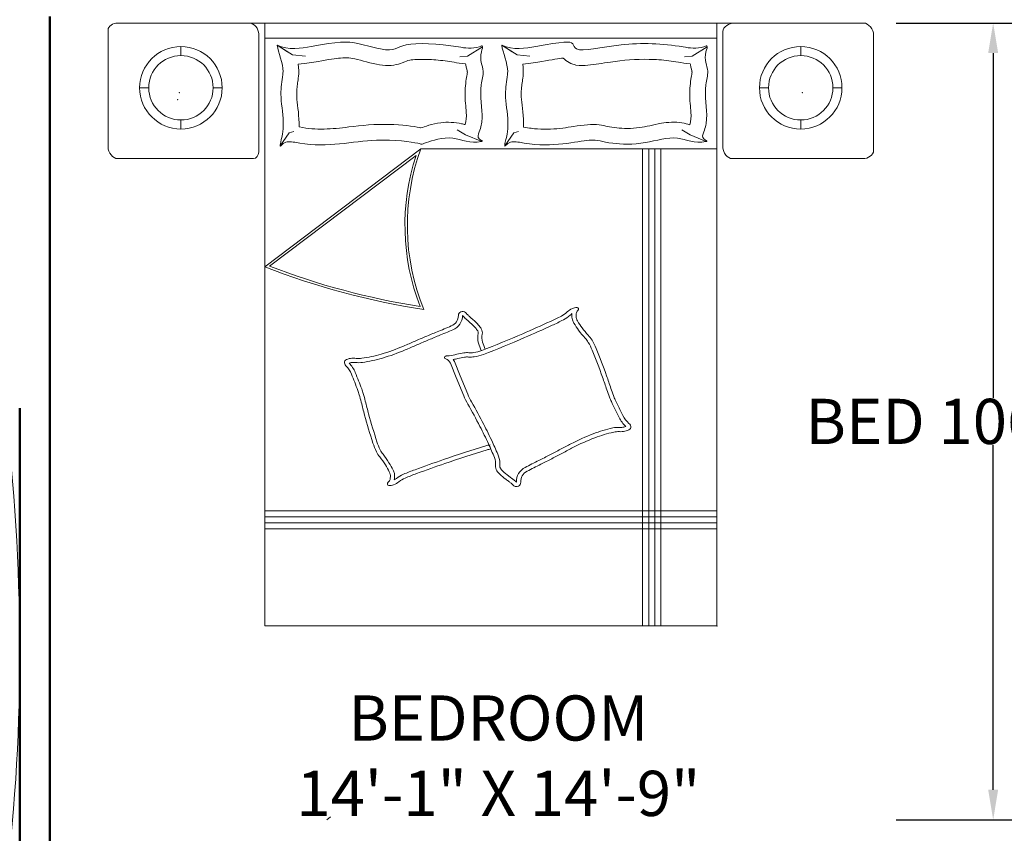
# Model space of a CAD drawing. Units: inches. Extents: x -466983 to 1020, y 324 to 318697.
# Tile 95 of 97: x 810 to 940, y 898 to 1006. Entities that reach past the tile are written whole.
import ezdxf

# ---------------------------------------------------------------- set-up
doc = ezdxf.new("R2010")
doc.units = ezdxf.units.IN
doc.header["$MEASUREMENT"] = 0
for name, color, linetype, lineweight in [('A-ANNO-DIMS', 2, 'Continuous', 18), ('A-AREA-IDEN', 7, 'Continuous', 25), ('A-FLOR-PATT', 252, 'Continuous', 13), ('A-FURN', 8, 'Continuous', 18), ('A-WALL', 7, 'Continuous', 50)]:
    doc.layers.add(name, color=color, linetype=linetype, lineweight=lineweight)
doc.styles.get("Standard").update_dxf_attribs({"font": 'arial.ttf'})
doc.dimstyles.get("Standard").update_dxf_attribs({"dimtxt": 6, "dimasz": 4, "dimexe": 3, "dimexo": 3, "dimgap": 0.09, "dimtad": 0, "dimtih": 1, "dimtoh": 1, "dimdec": 1, "dimzin": 0, "dimdsep": 46, "dimlunit": 3, "dimtxsty": 'Standard', "dimcen": 0.09, "dimadec": 0, "dimazin": 0, "dimtfac": 1, "dimtdec": 1, "dimtofl": 0, "dimtmove": 0, "dimatfit": 3, "dimfxl": 1, "dimtolj": 1, "dimtzin": 0, "dimarcsym": 0})

# ---------------------------------------------------------------- blocks, each defined once
blk = doc.blocks.new('A$C05F852CF')
for p, q in [((0.0306, 3.0783), (0.4692, 3.0783)), ((0.4692, 3.0783), (2.0768, 3.0783)), ((0.52, 3.0783), (0.52, 1.0783)), ((2.02, 3.0783), (2.02, 1.0783)), ((2.0768, 3.0783), (2.5066, 3.0783)), ((0, 3.0548), (0, 2.6659)), ((0.5, 3.0423), (0.5, 2.6496)), ((2.04, 3.05), (2.04, 2.6642)), ((2.54, 2.6547), (2.54, 3.0393)), ((0.52, 3.0283), (2.02, 3.0283)), ((0.2418, 2.9702), (0.2418, 3.0002)), ((0.5609, 3.0045), (0.5953, 2.9829)), ((0.5609, 3.0045), (0.6121, 2.9725)), ((1.2427, 2.9995), (1.1927, 2.9682)), ((2.2982, 2.9702), (2.2982, 3.0002)), ((0.6121, 2.9725), (0.6546, 2.9682)), ((1.1927, 2.9682), (1.1672, 2.9661)), ((0.1349, 2.8634), (0.1049, 2.8634)), ((0.3487, 2.8634), (0.3787, 2.8634)), ((2.1913, 2.8634), (2.1613, 2.8634)), ((2.4051, 2.8634), (2.4351, 2.8634)), ((0.2418, 2.7265), (0.2418, 2.7565)), ((2.2982, 2.7265), (2.2982, 2.7565)), ((0.5711, 2.6712), (0.6015, 2.7135)), ((0.6015, 2.7135), (0.6164, 2.7178)), ((1.1864, 2.7072), (1.1588, 2.7242)), ((1.2397, 2.6852), (1.1864, 2.7072)), ((1.0379, 2.6608), (0.52, 2.2697)), ((2.02, 2.6608), (1.0379, 2.6608)), ((1.7737, 2.6608), (1.7737, 1.0783)), ((1.7937, 2.6608), (1.7937, 1.0783)), ((1.8137, 2.6608), (1.8137, 1.0783)), ((1.8337, 2.6608), (1.8337, 1.0783)), ((0.0322, 2.6283), (0.4826, 2.6283)), ((2.0707, 2.6283), (2.5056, 2.6283)), ((0.52, 1.4597), (2.02, 1.4597)), ((0.52, 1.4397), (2.02, 1.4397)), ((0.52, 1.4197), (2.02, 1.4197)), ((0.52, 1.3997), (2.02, 1.3997)), ((0.52, 1.0783), (2.02, 1.0783)), ((0.726, 0.4346), (0.7377, 0.4444))]:
    blk.add_line(p, q)
for points in [[(1.3405, 2.9829), (1.306, 3.0045), (1.3573, 2.9725), (1.3998, 2.9682)], [(1.9879, 2.9995), (1.9379, 2.9682), (1.9124, 2.9661)], [(1.3162, 2.6712), (1.3467, 2.7135), (1.3616, 2.7178)], [(1.9848, 2.6852), (1.9315, 2.7072), (1.9039, 2.7242)]]:
    blk.add_lwpolyline(points)
for points in [[(1.0353, 2.1379, -0.173032), (1.022, 2.6388), (0.536, 2.2719, 0.053888)], [(1.7081, 1.7759, 0.101392), (1.7282, 1.7501, -0.223768), (1.7345, 1.736, -0.25558), (1.7315, 1.7308, -0.081563), (1.7151, 1.724, -0.071805), (1.6967, 1.7225, 0.069985), (1.6778, 1.7209, 0.03546), (1.6148, 1.7021, 0.029432), (1.5425, 1.6697, 0.001554), (1.5078, 1.6515, -0.00152), (1.4724, 1.6329, -0.004735), (1.4356, 1.6142, 0.00382), (1.3901, 1.5911, 0.296001), (1.3692, 1.5546, -0.649774), (1.3468, 1.5431, -0.02319), (1.3416, 1.5477, 0.0288), (1.3374, 1.5514, 0.005727), (1.3298, 1.557, -0.004358), (1.3198, 1.5645, -0.027528), (1.3001, 1.5812, -0.046214), (1.29, 1.5928, -0.194121), (1.2856, 1.6105, 0.133719), (1.2823, 1.6363, 0.011505), (1.2622, 1.682, 0.008882), (1.2338, 1.7401, 0.012426), (1.1937, 1.8139, -0.033612), (1.1801, 1.8418), (1.1552, 1.9026), (1.1361, 1.9495, 0.224341), (1.1204, 1.9638, -0.722772), (1.1202, 1.9734, -0.103513), (1.1242, 1.9739, 0.053465), (1.132, 1.9742, 0.030109), (1.1569, 1.9792, -0.031436), (1.1808, 1.984, -0.05324), (1.1971, 1.9844, 0.05518), (1.2128, 1.9849, 0.056271), (1.2402, 1.992, 0.0108), (1.3759, 2.0475, 0.00456), (1.4675, 2.0883, 0.01125), (1.5041, 2.106, 0.069394), (1.5235, 2.1196, -0.079756), (1.5405, 2.1311, -0.106399), (1.5562, 2.1345, -0.328642), (1.5608, 2.1312, -0.299547), (1.5587, 2.124, 0.189917), (1.5536, 2.1141, 0.033518), (1.5531, 2.1029, 0.075627), (1.554, 2.0981, 0.053489), (1.5579, 2.0898, 0.017838), (1.5727, 2.0672, 0.038394), (1.5932, 2.0425, -0.059529), (1.6058, 2.026, -0.035943), (1.6193, 1.9987, -0.011245), (1.6541, 1.9079, -0.006203), (1.6684, 1.8661, 0.010783), (1.6769, 1.8422, 0.019485), (1.6828, 1.8283, 0.005062)], [(1.6953, 1.7695, 0.098587), (1.7181, 1.7399, -0.040378), (1.7118, 1.7379, -0.071805), (1.6975, 1.7367, 0.069985), (1.6747, 1.7349, 0.03546), (1.6097, 1.7154, 0.029432), (1.5359, 1.6824, 0.001554), (1.5012, 1.6641, -0.00152), (1.4658, 1.6456, -0.004735), (1.4293, 1.627, 0.00382), (1.3835, 1.6038, 0.289814), (1.3549, 1.555, -0.018279), (1.3515, 1.5579, 0.0288), (1.3461, 1.5627, 0.005727), (1.3382, 1.5686, -0.004358), (1.3285, 1.5758, -0.027528), (1.31, 1.5916, -0.046214), (1.3016, 1.6012, -0.194121), (1.2997, 1.6085, 0.133719), (1.2955, 1.6417, 0.011505), (1.2752, 1.6881, 0.008882), (1.2465, 1.7466, 0.012426), (1.2061, 1.821, -0.033612), (1.1933, 1.8472), (1.1684, 1.908), (1.1493, 1.9549, 0.051417), (1.1455, 1.962, 0.017208), (1.1606, 1.9654, -0.031436), (1.1827, 1.9698, -0.05324), (1.196, 1.9702, 0.05518), (1.2149, 1.9708, 0.056271), (1.2453, 1.9787, 0.0108), (1.3816, 2.0344, 0.00456), (1.4734, 2.0753, 0.01125), (1.5106, 2.0933, 0.069394), (1.5332, 2.1091, -0.038161), (1.5392, 2.114, 0.029361), (1.5389, 2.1025, 0.075627), (1.5405, 2.0934, 0.053489), (1.5457, 2.0824, 0.017838), (1.5611, 2.0589, 0.038394), (1.583, 2.0326, -0.059529), (1.5935, 2.0187, -0.035943), (1.6061, 1.9933, -0.011245), (1.6406, 1.9031, -0.006203), (1.6549, 1.8617, 0.010783), (1.6635, 1.8371, 0.019485), (1.6699, 1.8222, 0.005062)]]:
    blk.add_lwpolyline(points, format="xyb", close=True)
for points in [[(1.27, 1.665, 0.025626), (1.2575, 1.662, 0.0108), (1.1179, 1.617, 0.00456), (1.0234, 1.5834, 0.01125), (0.9856, 1.5685, 0.069394), (0.9653, 1.5565, -0.079756), (0.9474, 1.5464, -0.106399), (0.9315, 1.5441, -0.328642), (0.9272, 1.5478, -0.299547), (0.9298, 1.5548, 0.189917), (0.9357, 1.5643, 0.033518), (0.9369, 1.5754, 0.075627), (0.9364, 1.5803, 0.053489), (0.9332, 1.5888, 0.017838), (0.9202, 1.6125, 0.038394), (0.9016, 1.6387, -0.059529), (0.8903, 1.6561, -0.035943), (0.8789, 1.6844, -0.011245), (0.8512, 1.7776, -0.006203), (0.8402, 1.8203, 0.010783), (0.8336, 1.8448, 0.019485), (0.8287, 1.8592, 0.005062), (0.8076, 1.9133, 0.101392), (0.7895, 1.9406, -0.223768), (0.7843, 1.9551, -0.25558), (0.7876, 1.9601, -0.081563), (0.8046, 1.9656, -0.071805), (0.823, 1.9657, 0.069985), (0.842, 1.9658, 0.03546), (0.9062, 1.9798, 0.029432), (0.9807, 2.0065, 0.001554), (1.0167, 2.022, -0.00152), (1.0535, 2.0378, -0.004735), (1.0916, 2.0536, 0.00382), (1.1388, 2.0731, 0.296001), (1.1624, 2.108, -0.649774), (1.1856, 2.1178, -0.02319), (1.1904, 2.1128, 0.0288), (1.1944, 2.1088, 0.005727), (1.2015, 2.1025, -0.004358), (1.2108, 2.0944, -0.027528), (1.2292, 2.0762, -0.046214), (1.2384, 2.0638, -0.194121), (1.2414, 2.0458, 0.133719), (1.2427, 2.0199, 0.005779), (1.2507, 1.9961)], [(1.2674, 1.6787, 0.025626), (1.2535, 1.6753, 0.0108), (1.1134, 1.6301, 0.00456), (1.0187, 1.5964, 0.01125), (0.9802, 1.5813, 0.069394), (0.9566, 1.5673, -0.042175), (0.9495, 1.5626, 0.031457), (0.9508, 1.5747, 0.075627), (0.9499, 1.5838, 0.053489), (0.9456, 1.595, 0.017838), (0.9321, 1.6196, 0.038394), (0.9123, 1.6476, -0.059529), (0.9028, 1.6622, -0.035943), (0.8922, 1.6886, -0.011245), (0.8646, 1.7812, -0.006203), (0.8536, 1.8236, 0.010783), (0.8469, 1.8487, 0.019485), (0.8417, 1.8641, 0.005062), (0.8204, 1.9185, 0.100237), (0.7996, 1.9501, -0.044209), (0.8066, 1.9519, -0.071805), (0.8211, 1.952, 0.069985), (0.8439, 1.9521, 0.03546), (0.9101, 1.9665, 0.029432), (0.9862, 1.9937, 0.001554), (1.0222, 2.0093, -0.00152), (1.0589, 2.025, -0.004735), (1.0968, 2.0408, 0.00382), (1.1442, 2.0604, 0.294287), (1.1763, 2.1074, -0.02184), (1.18, 2.1036, 0.0288), (1.1851, 2.0984, 0.005727), (1.1924, 2.092, -0.004358), (1.2016, 2.084, -0.027528), (1.2189, 2.0669, -0.046214), (1.2266, 2.0566, -0.194121), (1.2279, 2.0488, 0.133719), (1.2295, 2.0156, 0.005779), (1.2376, 1.9915, 0.005779)]]:
    blk.add_lwpolyline(points, format="xyb")
for centre, radius in [((0.2418, 2.8634), 0.1369), ((2.2982, 2.8634), 0.1369), ((0.2418, 2.8634), 0.1069), ((2.2982, 2.8634), 0.1069)]:
    blk.add_circle(centre, radius)
for centre, radius, start, end in [((1.7308, 2.407), 0.7379, 159.8846, 202.2194), ((1.4058, 4.5145), 2.4132, 248.4641, 261.4655)]:
    blk.add_arc(centre, radius, start, end)
for points in [[(0, 3.0548), (0, 3.0677), (0.0177, 3.0783), (0.0306, 3.0783)], [(0.5, 3.0423), (0.5, 3.0581), (0.485, 3.0783), (0.4692, 3.0783)], [(2.04, 3.05), (2.04, 3.0655), (2.0613, 3.0783), (2.0768, 3.0783)], [(2.5066, 3.0783), (2.5237, 3.0783), (2.54, 3.0564), (2.54, 3.0393)], [(0.0322, 2.6283), (0.0157, 2.6283), (0, 2.6494), (0, 2.6659)], [(0.5, 2.6496), (0.5, 2.6405), (0.4918, 2.6283), (0.4826, 2.6283)], [(2.04, 2.6642), (2.04, 2.6485), (2.055, 2.6283), (2.0707, 2.6283)], [(2.5056, 2.6283), (2.5201, 2.6283), (2.54, 2.6403), (2.54, 2.6547)]]:
    blk.add_open_spline(points, degree=3)
for points, knots in [([(0.5609, 3.0045), (0.565, 2.9818), (0.5836, 2.9366), (0.5776, 2.889), (0.5689, 2.8351), (0.5832, 2.7709), (0.5808, 2.7088), (0.5744, 2.6927), (0.5693, 2.6651), (0.5803, 2.6793), (0.5989, 2.6876), (0.7172, 2.6598), (0.8681, 2.7029), (1.0484, 2.6781), (1.0324, 2.6731), (1.1431, 2.7116), (1.202, 2.6757), (1.2459, 2.6867), (1.2222, 2.695), (1.2359, 2.7251), (1.2468, 2.781), (1.2288, 2.8492), (1.2515, 2.925), (1.2279, 2.9609), (1.2471, 3.0058), (1.2098, 2.9902), (1.1177, 3.0095), (0.956, 3.0159), (0.9532, 2.9758), (0.7999, 3.021), (0.7569, 3.0151), (0.5986, 2.9869), (0.561, 3.0049)], [16.816032, 16.816032, 16.816032, 16.816032, 79.038845, 88.513895, 147.565266, 227.196862, 259.685448, 283.955301, 296.511304, 302.432558, 320.230942, 354.322559, 575.279549, 734.72356, 845.740421, 943.033103, 1029.533967, 1032.845074, 1043.313584, 1065.311534, 1104.921835, 1208.53002, 1248.510714, 1303.102727, 1321.01326, 1329.647833, 1389.371624, 1571.817644, 1750.274161, 1823.189073, 1967.937033, 2020.912329, 2020.912329, 2020.912329, 2020.912329]), ([(1.306, 3.0045), (1.3102, 2.9818), (1.3287, 2.9366), (1.3228, 2.889), (1.314, 2.8351), (1.3284, 2.7709), (1.3259, 2.7088), (1.3196, 2.6927), (1.3144, 2.6651), (1.3254, 2.6793), (1.3441, 2.6876), (1.4624, 2.6598), (1.6132, 2.7029), (1.6436, 2.6781), (1.7775, 2.6731), (1.8882, 2.7116), (1.9472, 2.6757), (1.9911, 2.6867), (1.9673, 2.695), (1.981, 2.7251), (1.992, 2.781), (1.974, 2.8492), (1.9967, 2.925), (1.9731, 2.9609), (1.9922, 3.0058), (1.9549, 2.9902), (1.8628, 3.0095), (1.7011, 3.0159), (1.5483, 2.9758), (1.5451, 3.021), (1.5021, 3.0151), (1.3437, 2.9869), (1.3062, 3.0049)], [16.816032, 16.816032, 16.816032, 16.816032, 79.038845, 88.513895, 147.565266, 227.196862, 259.685448, 283.955301, 296.511304, 302.432558, 320.230942, 354.322559, 575.279549, 734.72356, 845.740421, 943.033103, 1029.533967, 1032.845074, 1043.313584, 1065.311534, 1104.921835, 1208.53002, 1248.510714, 1303.102727, 1321.01326, 1329.647833, 1389.371624, 1571.817644, 1750.274161, 1823.189073, 1967.937033, 2020.912329, 2020.912329, 2020.912329, 2020.912329]), ([(0.631, 2.9418), (0.6332, 2.9288), (0.633, 2.9104), (0.6308, 2.893), (0.6298, 2.8865), (0.628, 2.8726), (0.6273, 2.866), (0.6257, 2.8474), (0.6257, 2.8375), (0.629, 2.8013), (0.6345, 2.7696), (0.6337, 2.7333)], [67.285362, 67.285362, 67.285362, 67.285362, 87.399558, 87.399558, 107.513754, 107.513754, 127.62795, 127.62795, 167.856341, 167.856341, 238.127268, 238.127268, 238.127268, 238.127268]), ([(1.186, 2.943), (1.1557, 2.9456), (1.1387, 2.9502), (1.0976, 2.9551), (1.0776, 2.9567), (1.0342, 2.9582), (1.0123, 2.957), (0.991, 2.9533), (0.9902, 2.9517), (0.962, 2.9403), (0.9371, 2.935), (0.8851, 2.9413), (0.8522, 2.9513), (0.8033, 2.9629), (0.7938, 2.964), (0.755, 2.9608), (0.7319, 2.9572), (0.6794, 2.9481), (0.658, 2.9434), (0.631, 2.9418)], [1364.380335, 1364.380335, 1364.380335, 1364.380335, 1423.60231, 1423.60231, 1482.824284, 1482.824284, 1566.205036, 1566.205036, 1649.585789, 1649.585789, 1732.966542, 1732.966542, 1816.347295, 1816.347295, 1899.728048, 1899.728048, 1960.499853, 1960.499853, 1990.525565, 1990.525565, 1990.525565, 1990.525565]), ([(1.1845, 2.7412), (1.189, 2.7552), (1.1894, 2.765), (1.1874, 2.7998), (1.1843, 2.8219), (1.1844, 2.8664), (1.1882, 2.8901), (1.192, 2.9105), (1.1922, 2.9144), (1.1921, 2.9158), (1.1908, 2.9212), (1.1875, 2.9351), (1.1867, 2.9388), (1.186, 2.943)], [1072.516901, 1072.516901, 1072.516901, 1072.516901, 1129.100964, 1129.100964, 1185.685027, 1185.685027, 1226.035089, 1226.035089, 1249.281274, 1249.281274, 1272.52746, 1272.52746, 1279.689275, 1279.689275, 1279.689275, 1279.689275]), ([(1.3759, 2.942), (1.3781, 2.929), (1.378, 2.9106), (1.3757, 2.893), (1.3748, 2.8866), (1.373, 2.8727), (1.3722, 2.8661), (1.3706, 2.8475), (1.3707, 2.8375), (1.3739, 2.8012), (1.3795, 2.7694), (1.3787, 2.7331)], [67.156228, 67.156228, 67.156228, 67.156228, 87.297212, 87.297212, 107.438196, 107.438196, 127.57918, 127.57918, 167.861148, 167.861148, 238.25357, 238.25357, 238.25357, 238.25357]), ([(1.5104, 2.9621), (1.4964, 2.9606), (1.4732, 2.9568), (1.4226, 2.948), (1.4017, 2.9435), (1.3759, 2.942)], [1904.3965, 1904.3965, 1904.3965, 1904.3965, 1961.927876, 1961.927876, 1990.619445, 1990.619445, 1990.619445, 1990.619445]), ([(1.9314, 2.9432), (1.8997, 2.9459), (1.8822, 2.9507), (1.8387, 2.9557), (1.8168, 2.9572), (1.7515, 2.9587), (1.7088, 2.9551), (1.6403, 2.9447), (1.6154, 2.9402), (1.5795, 2.937), (1.5675, 2.9361), (1.5394, 2.9412), (1.5201, 2.9507), (1.5104, 2.9621)], [1364.265661, 1364.265661, 1364.265661, 1364.265661, 1426.240795, 1426.240795, 1488.215928, 1488.215928, 1612.166195, 1612.166195, 1689.92864, 1689.92864, 1733.064362, 1733.064362, 1768.978829, 1768.978829, 1768.978829, 1768.978829]), ([(1.9299, 2.7409), (1.9344, 2.755), (1.9348, 2.7648), (1.9328, 2.7996), (1.9297, 2.8217), (1.9298, 2.8662), (1.9336, 2.8899), (1.9374, 2.9105), (1.9376, 2.9144), (1.9375, 2.9159), (1.9362, 2.9214), (1.9329, 2.9353), (1.9321, 2.939), (1.9314, 2.9432)], [1072.238498, 1072.238498, 1072.238498, 1072.238498, 1128.864869, 1128.864869, 1185.491239, 1185.491239, 1225.989553, 1225.989553, 1249.326401, 1249.326401, 1272.66325, 1272.66325, 1279.788508, 1279.788508, 1279.788508, 1279.788508]), ([(1.0381, 2.7304), (1.0497, 2.7345), (1.0742, 2.7435), (1.1251, 2.7504), (1.1528, 2.749), (1.1769, 2.7432), (1.1809, 2.7421), (1.1845, 2.7412)], [843.64503, 843.64503, 843.64503, 843.64503, 911.27572, 911.27572, 959.088062, 959.088062, 969.47998, 969.47998, 969.47998, 969.47998]), ([(1.3787, 2.7331), (1.3984, 2.7296), (1.4106, 2.7278), (1.4401, 2.7258), (1.4545, 2.7258), (1.4962, 2.7276), (1.5219, 2.7313), (1.5767, 2.7399), (1.6067, 2.7436), (1.6527, 2.7371), (1.662, 2.7326), (1.7084, 2.7282), (1.7364, 2.7276), (1.7849, 2.734), (1.8076, 2.7406), (1.8563, 2.7489), (1.8812, 2.7508), (1.914, 2.7451), (1.9226, 2.7428), (1.9299, 2.7409)], [345.267918, 345.267918, 345.267918, 345.267918, 387.167414, 387.167414, 429.06691, 429.06691, 512.865903, 512.865903, 629.317545, 629.317545, 745.769188, 745.769188, 834.622813, 834.622813, 901.414409, 901.414409, 948.921878, 948.921878, 969.679511, 969.679511, 969.679511, 969.679511]), ([(0.6337, 2.7333), (0.6515, 2.7301), (0.6627, 2.7284), (0.6898, 2.7263), (0.7032, 2.726), (0.7436, 2.727), (0.7707, 2.73), (0.8409, 2.7383), (0.8881, 2.7432), (0.9755, 2.7406), (1.0125, 2.7357), (1.0356, 2.7309), (1.0369, 2.7307), (1.0381, 2.7304)], [345.4047, 345.4047, 345.4047, 345.4047, 383.386056, 383.386056, 421.367413, 421.367413, 497.330126, 497.330126, 611.561469, 611.561469, 725.792813, 725.792813, 732.434768, 732.434768, 732.434768, 732.434768])]:
    blk.add_open_spline(points, degree=3, knots=knots)
for p in [(0.2366, 2.8475), (2.3034, 2.8475), (0.2309, 2.8244), (2.02, 1.0783), (2.02, 1.0783)]:
    blk.add_point(p)
blk = doc.blocks.new('L Shaped Sofa')
at = {"ltscale": 2}
blk.add_arc((2416.36, 1205.03), 481.82, 262.8867, 276.632, dxfattribs=at)
blk = doc.blocks.new('*D73')
at = {"layer": 'A-ANNO-DIMS', "color": 0, "lineweight": -2, "transparency": 16777216}
for p, q in [((926.13, 1005.06), (942, 1005.06)), ((939, 1001.06), (939, 955.34)), ((939, 903.32), (939, 949.04)), ((926.13, 899.32), (942, 899.32))]:
    blk.add_line(p, q, dxfattribs=at)
at = {"layer": 'A-ANNO-DIMS', "color": 0, "transparency": 16777216}
for points in [[(938.33, 1001.06), (939.66, 1001.06), (939, 1005.06)], [(938.33, 903.32), (939.66, 903.32), (939, 899.32)]]:
    blk.add_solid(points, dxfattribs=at)
at = {"layer": 'Defpoints', "color": 0, "transparency": 16777216}
for p in [(923.13, 1005.06), (939, 1005.06), (923.13, 899.32)]:
    blk.add_point(p, dxfattribs=at)
at = {"layer": 'A-ANNO-DIMS', "color": 0, "transparency": 16777216, "insert": (939, 952.19), "char_height": 6, "attachment_point": 5}
blk.add_mtext('\\A1;BED 106 TYP.', dxfattribs=at)
blk = doc.blocks.new('*D74')
at = {"layer": 'A-ANNO-DIMS', "color": 0, "lineweight": -2, "transparency": 16777216}
for p, q in [((821.53, 896.32), (821.53, 880.45)), ((923.13, 896.32), (923.13, 880.45)), ((825.53, 883.45), (855.59, 883.45)), ((919.13, 883.45), (889.08, 883.45))]:
    blk.add_line(p, q, dxfattribs=at)
at = {"layer": 'A-ANNO-DIMS', "color": 0, "transparency": 16777216}
for points in [[(825.53, 884.12), (825.53, 882.79), (821.53, 883.45)], [(919.13, 884.12), (919.13, 882.79), (923.13, 883.45)]]:
    blk.add_solid(points, dxfattribs=at)
at = {"layer": 'Defpoints', "color": 0, "transparency": 16777216}
for p in [(821.53, 899.32), (923.13, 899.32), (923.13, 883.45)]:
    blk.add_point(p, dxfattribs=at)
at = {"layer": 'A-ANNO-DIMS', "color": 0, "transparency": 16777216, "insert": (872.33, 883.45), "char_height": 6, "attachment_point": 5}
blk.add_mtext('\\A1;102 TYP.', dxfattribs=at)

msp = doc.modelspace()

# ---------------------------------------------------------------- hatches: boundary and pattern name
at = {"layer": 'A-FLOR-PATT', "transparency": 33554572}
h = msp.add_hatch(dxfattribs=at)
h.set_pattern_fill('ANSI37', color=256, scale=30)
h.set_pattern_definition([(45, (-1212.4137, -290.035), (-2.6516504, 2.6516504), []), (135, (-1212.4137, -290.035), (-2.6516504, -2.6516504), [])])
h.paths.add_polyline_path([(901.81, 1075.94), (900.61, 1075.94), (900.61, 1065.39), (899.39, 1065.39), (898.09, 1065.39), (892.84, 1058.71, -0.258377), (892.19, 1058.35), (879.98, 1058.35, -0.20177), (879.44, 1058.58), (874.08, 1065.39), (872.78, 1065.39), (871.56, 1065.39), (871.56, 1075.94), (813.81, 1075.94), (813.81, 1044.79), (832.39, 1044.79, -0.394795), (848.66, 1028.54), (848.66, 1009.94), (901.81, 1009.94), (901.81, 1015.94), (901.31, 1015.94), (871.31, 1015.94), (871.31, 1017.25), (871.33, 1017.25, -0.401453), (901.31, 1045.94), (901.81, 1045.94)])
edge = h.paths.add_edge_path(flags=16)
edge.add_line((847.77, 1068.95), (847.77, 1073.71))
edge.add_arc((849.23, 1073.71), 1.45, 90, 180, ccw=False)
edge.add_line((849.23, 1075.16), (864.49, 1075.16))
edge.add_arc((864.49, 1073.71), 1.45, 0, 90, ccw=False)
edge.add_line((865.95, 1073.71), (865.95, 1069))
edge.add_arc((832.64, 1068.98), 33.3, -20.6123, 0.0472, ccw=False)
edge.add_ellipse((856.86, 1058.48), major_axis=(0, 10.21), ratio=0.685919, start_angle=100.0088, end_angle=259.9912, ccw=False)
edge.add_arc((881.07, 1068.98), 33.3, 180.0472, 200.6123, ccw=False)
h.paths.add_polyline_path([(853.15, 1066.48), (853.15, 1066.45), (853.15, 1066.45, 0.433107), (852.92, 1066.68), (852.92, 1066.45), (853.15, 1066.45), (853.15, 1066.48), (853.09, 1066.61, 0.697939), (852.7, 1066.45), (852.7, 1066.45), (852.7, 1066.48), (852.92, 1067), (852.92, 1066.68, -0.396254)], flags=0)
h.paths.add_polyline_path([(861.02, 1066.48), (861.02, 1066.45), (861.02, 1066.45, 0.416404), (860.8, 1066.68), (860.8, 1066.45), (861.02, 1066.45), (861.02, 1066.48), (860.97, 1066.61, 0.713344), (860.57, 1066.45), (860.57, 1066.45), (860.57, 1066.48), (860.8, 1067), (860.8, 1066.68, -0.379973)], flags=0)
edge = h.paths.add_edge_path(flags=0)
edge.add_spline(control_points=[(861.13, 1065.79), (861.47, 1065.25), (861.61, 1065.02), (861.98, 1064.37), (862.19, 1063.94), (862.56, 1063.04), (862.72, 1062.56), (862.99, 1061.58), (863.09, 1061.07), (863.25, 1060.03), (863.29, 1059.5), (863.33, 1058.44), (863.32, 1057.91), (863.24, 1056.85), (863.17, 1056.33), (862.97, 1055.31), (862.84, 1054.81), (862.54, 1053.85), (862.36, 1053.39), (861.95, 1052.52), (861.73, 1052.12), (861.23, 1051.36), (860.97, 1051.02), (860.4, 1050.39), (860.11, 1050.12), (859.49, 1049.65), (859.18, 1049.45), (858.53, 1049.13), (858.2, 1049.01), (857.53, 1048.85), (857.2, 1048.81), (856.52, 1048.81), (856.19, 1048.85), (855.52, 1049.01), (855.19, 1049.13), (854.54, 1049.45), (854.23, 1049.64), (853.61, 1050.12), (853.32, 1050.39), (852.75, 1051.01), (852.49, 1051.36), (852, 1052.11), (851.77, 1052.52), (851.36, 1053.39), (851.18, 1053.85), (850.88, 1054.81), (850.75, 1055.31), (850.55, 1056.33), (850.48, 1056.85), (850.4, 1057.9), (850.39, 1058.44), (850.43, 1059.5), (850.47, 1060.03), (850.63, 1061.07), (850.73, 1061.58), (851, 1062.56), (851.16, 1063.04), (851.53, 1063.94), (851.73, 1064.37), (852.11, 1065.02), (852.25, 1065.25), (852.61, 1065.73)], knot_values=[3.915332, 3.915332, 3.915332, 3.915332, 4.013468, 4.013468, 4.175532, 4.175532, 4.337596, 4.337596, 4.49966, 4.49966, 4.661724, 4.661724, 4.823788, 4.823788, 4.985852, 4.985852, 5.147916, 5.147916, 5.30998, 5.30998, 5.472044, 5.472044, 5.634109, 5.634109, 5.796173, 5.796173, 5.958237, 5.958237, 6.120301, 6.120301, 6.282365, 6.282365, 6.444429, 6.444429, 6.606493, 6.606493, 6.768557, 6.768557, 6.930621, 6.930621, 7.092685, 7.092685, 7.254749, 7.254749, 7.416813, 7.416813, 7.578878, 7.578878, 7.740942, 7.740942, 7.903006, 7.903006, 8.06507, 8.06507, 8.227134, 8.227134, 8.389198, 8.389198, 8.551262, 8.551262, 8.65037, 8.65037, 8.65037, 8.65037], degree=3, periodic=0)
edge.add_line((852.64, 1065.79), (861.13, 1065.79))
edge = h.paths.add_edge_path(flags=0)
edge.add_ellipse((856.85, 1057.74), major_axis=(0, 7.79), ratio=0.687861, start_angle=0, end_angle=360)
h.paths.add_polyline_path([(848.86, 1069.39), (848.86, 1073.96, -0.414214), (849.95, 1075.05), (863.77, 1075.05, -0.414214), (864.86, 1073.96), (864.86, 1069.39, -0.388936), (864.52, 1069.03, -0.043561), (849.2, 1069.03, -0.388936)], flags=0)
h.paths.add_polyline_path([(853.1, 1068.11, -1), (852.68, 1068.11, -1)], flags=0)
edge = h.paths.add_edge_path(flags=0)
edge.add_ellipse((856.86, 1057.34), major_axis=(0, 2.21), ratio=0.657164, start_angle=0, end_angle=360)
h.paths.add_polyline_path([(861.04, 1068.11, -1), (860.62, 1068.11, -1)], flags=0)
edge = h.paths.add_edge_path()
edge.add_line((573.95, 1057.34), (573.95, 1075.94))
edge.add_line((573.95, 1075.94), (558.73, 1075.94))
edge.add_line((558.73, 1075.94), (558.73, 1065.39))
edge.add_line((558.73, 1065.39), (557.51, 1065.39))
edge.add_line((557.51, 1065.39), (556.21, 1065.39))
edge.add_line((556.21, 1065.39), (550.95, 1058.71))
edge.add_arc((550.3, 1059.12), 0.765, 270, 327.9483, ccw=False)
edge.add_line((550.3, 1058.35), (538.1, 1058.35))
edge.add_arc((538.1, 1059.12), 0.765, 224.3704, 270, ccw=False)
edge.add_line((537.55, 1058.58), (532.2, 1065.39))
edge.add_line((532.2, 1065.39), (530.9, 1065.39))
edge.add_line((530.9, 1065.39), (529.67, 1065.39))
edge.add_line((529.67, 1065.39), (529.67, 1075.94))
edge.add_line((529.67, 1075.94), (520.81, 1075.94))
edge.add_line((520.81, 1075.94), (520.81, 1045.94))
edge.add_line((520.81, 1045.94), (521.31, 1045.94))
edge.add_arc((521.31, 1015.94), 30, 2.5075, 90, ccw=False)
edge.add_line((551.28, 1017.25), (551.31, 1017.25))
edge.add_line((551.31, 1017.25), (551.31, 1015.94))
edge.add_line((551.31, 1015.94), (520.81, 1015.94))
edge.add_line((520.81, 1015.94), (520.81, 1009.94))
edge.add_line((520.81, 1009.94), (559.19, 1010.4))
edge.add_arc((559.19, 1011.86), 1.45, 180, 270, ccw=False)
edge.add_line((557.74, 1011.86), (557.74, 1016.56))
edge.add_arc((591.04, 1016.59), 33.3, 159.3877, 180.0472, ccw=False)
edge.add_ellipse((566.82, 1027.08), major_axis=(0, 10.21), ratio=0.685919, start_angle=280.0088, end_angle=439.9912, ccw=False)
edge.add_arc((542.61, 1016.59), 33.3, 0.0472, 20.6123, ccw=False)
edge.add_line((575.91, 1016.62), (575.91, 1011.86))
edge.add_arc((574.46, 1011.86), 1.45, -90, 0, ccw=False)
edge.add_line((574.46, 1010.4), (608.81, 1009.94))
edge.add_line((608.81, 1009.94), (608.81, 1041.09))
edge.add_line((608.81, 1041.09), (590.22, 1041.09))
edge.add_arc((590.78, 1057.91), 16.83, 181.9277, 268.1032, ccw=False)
edge = h.paths.add_edge_path()
edge.add_ellipse((494.24, 583.62), major_axis=(0, 10.21), ratio=0.685919, start_angle=280.0088, end_angle=439.9912, ccw=False)
edge.add_arc((470.03, 573.12), 33.3, 0.0472, 20.6123, ccw=False)
edge.add_line((503.33, 573.15), (503.33, 568.39))
edge.add_arc((501.88, 568.39), 1.45, -90, 0, ccw=False)
edge.add_line((501.88, 566.94), (539.81, 566.94))
edge.add_line((539.81, 566.94), (539.81, 572.94))
edge.add_line((539.81, 572.94), (539.31, 572.94))
edge.add_line((539.31, 572.94), (509.31, 572.94))
edge.add_line((509.31, 572.94), (509.31, 574.25))
edge.add_line((509.31, 574.25), (509.33, 574.25))
edge.add_arc((539.31, 572.94), 30, 90, 177.4925, ccw=False)
edge.add_line((539.31, 602.94), (539.81, 602.94))
edge.add_line((539.81, 602.94), (539.81, 626.94))
edge.add_line((539.81, 626.94), (531.77, 626.94))
edge.add_line((531.77, 626.94), (531.77, 616.39))
edge.add_line((531.77, 616.39), (530.55, 616.39))
edge.add_line((530.55, 616.39), (529.25, 616.39))
edge.add_line((529.25, 616.39), (523.71, 609.35))
edge.add_line((523.71, 609.35), (510.78, 609.35))
edge.add_line((510.78, 609.35), (505.24, 616.39))
edge.add_line((505.24, 616.39), (503.94, 616.39))
edge.add_line((503.94, 616.39), (502.72, 616.39))
edge.add_line((502.72, 616.39), (502.72, 626.94))
edge.add_line((502.72, 626.94), (481.7, 626.94))
edge.add_line((481.7, 626.94), (481.7, 611))
edge.add_arc((467.27, 611.47), 14.44, 271.9277, 358.1032, ccw=False)
edge.add_line((467.76, 597.05), (451.81, 597.05))
edge.add_line((451.81, 597.05), (451.81, 584.4))
edge.add_line((451.81, 584.4), (451.81, 566.94))
edge.add_line((451.81, 566.94), (486.61, 566.94))
edge.add_arc((486.61, 568.39), 1.45, 180, 270, ccw=False)
edge.add_line((485.16, 568.39), (485.16, 573.1))
edge.add_arc((518.46, 573.12), 33.3, 159.3877, 180.0472, ccw=False)
h.paths.add_polyline_path([(836.26, 1020.73), (879.89, 1020.73), (879.89, 1039.39), (836.26, 1039.39)], flags=25)
h.paths.add_polyline_path([(549.99, 1036.75), (593.61, 1036.75), (593.61, 1055.41), (549.99, 1055.41)], flags=24)
h.paths.add_polyline_path([(475.12, 595.6), (518.75, 595.6), (518.75, 614.25), (475.12, 614.25)], flags=24)
h = msp.add_hatch(dxfattribs=at)
h.set_pattern_fill('ANSI37', color=256, scale=20)
h.set_pattern_definition([(45, (-1212.4137, -290.035), (-1.767767, 1.767767), []), (135, (-1212.4137, -290.035), (-1.767767, -1.767767), [])])
h.paths.add_polyline_path([(809.81, 870.94), (809.81, 888.15), (807, 888.15), (802.66, 888.15), (789.38, 888.15), (786.28, 888.15, -0.414214), (785.5, 888.94), (785.5, 900.2), (785.5, 908.47, -0.414214), (786.81, 909.78, -0.414214), (785.5, 911.09), (785.5, 929.1, -0.414214), (786.81, 930.41, -0.414214), (785.5, 931.72), (785.5, 931.9, -0.414214), (784.19, 930.59), (766.72, 930.59, -0.412359), (765.41, 931.9, -0.413741), (764.11, 930.58), (744.58, 930.42, -0.416556), (743.79, 931.21), (743.79, 933.52), (742.22, 933.52), (742.22, 952.02, -0.001344), (743.79, 952.2), (743.79, 953.94), (678.59, 953.94), (678.59, 951.13), (678.59, 946.79), (678.59, 933.52), (678.59, 930.42, -0.414214), (677.81, 929.63), (666.55, 929.63), (658.27, 929.63, -0.414214), (656.96, 930.94, -0.414214), (655.66, 929.63), (637.64, 929.63, -0.414214), (636.33, 930.94, -0.414214), (635.02, 929.63), (634.84, 929.63, -0.414214), (636.15, 928.32), (636.15, 910.85, -0.412359), (634.85, 909.55, -0.413741), (636.17, 908.25), (636.32, 888.71, -0.416556), (635.54, 887.92), (633.23, 887.92), (633.23, 886.35), (614.72, 886.35, -0.001344), (614.54, 887.92), (612.81, 887.92), (612.81, 834.94), (612.81, 752.94), (612.81, 748.94), (612.81, 697.94), (654.81, 697.94), (654.81, 701.94), (715.81, 701.94), (715.81, 737.44), (774.29, 737.44), (774.29, 795.94), (809.81, 795.94)])
h.paths.add_polyline_path([(679.28, 849.58, 0.102523), (682.15, 849.26, -0.080461), (694.54, 849.77, -0.283899), (694.48, 849.01, 0.136605), (694.41, 848.81, -0.030441), (694.54, 846.89), (694.54, 842.62), (694.54, 838.35, -0.028219), (694.42, 836.57), (694.43, 836.57, 0.196187), (694.45, 836.27, -0.302897), (694.54, 835.47, -0.080461), (682.15, 835.98, 0.102523), (679.28, 835.66, -0.58611), (678.65, 836.02), (678.65, 849.22, -0.58611)], flags=16)
h.paths.add_polyline_path([(679.52, 848.65, 0.699597), (679.48, 848.63, 1.20716), (679.19, 848.74, 0.010621)], flags=0)
h.paths.add_polyline_path([(679.49, 836.56, -0.013798), (679.92, 836.66, -0.071703), (682.85, 837.14, -0.165743), (682.17, 839.1), (682.17, 842.61), (682.17, 846.06, -0.240616), (683.47, 848.68, -0.068263), (693.93, 849.01), (693.79, 848.71), (693.79, 849.02, 0.067332), (683.47, 848.68, 0.240616), (682.17, 846.06), (682.17, 842.61), (682.17, 839.1, 0.23459), (683.46, 836.55, 0.068093), (693.79, 836.2), (693.79, 836.51), (693.93, 836.21, -0.077215), (682.24, 836.78, 0.086627), (679.53, 836.57, -0.628402), (679.5, 836.57), (679.5, 836.61, 0.910458)], flags=0)
h.paths.add_polyline_path([(679.48, 848.64), (679.21, 848.65), (679.21, 836.57, 0.913566), (679.36, 836.59), (679.48, 836.58)], flags=0)
h.paths.add_polyline_path([(679.28, 829.86, 0.102523), (682.15, 829.55, -0.080461), (694.54, 830.06, -0.283899), (694.48, 829.29, 0.136605), (694.41, 829.1, -0.030441), (694.54, 827.18), (694.54, 822.9), (694.54, 818.63, -0.028219), (694.42, 816.85), (694.43, 816.85, 0.196187), (694.45, 816.56, -0.302897), (694.54, 815.75, -0.080461), (682.15, 816.26, 0.102523), (679.28, 815.95, -0.58611), (678.65, 816.3), (678.65, 829.51, -0.58611)], flags=16)
h.paths.add_polyline_path([(679.52, 828.94, 0.699597), (679.48, 828.92, 1.20716), (679.19, 829.03, 0.010621)], flags=0)
h.paths.add_polyline_path([(679.49, 816.85, -0.013798), (679.92, 816.94, -0.071703), (682.85, 817.43, -0.165743), (682.17, 819.39), (682.17, 822.89), (682.17, 826.34, -0.240616), (683.47, 828.96, -0.068263), (693.93, 829.29), (693.79, 828.99), (693.79, 829.31, 0.067332), (683.47, 828.96, 0.240616), (682.17, 826.34), (682.17, 822.89), (682.17, 819.39, 0.23459), (683.46, 816.84, 0.068093), (693.79, 816.48), (693.79, 816.8), (693.93, 816.49, -0.077215), (682.24, 817.07, 0.086627), (679.53, 816.85, -0.628402), (679.5, 816.86), (679.5, 816.89, 0.910458)], flags=0)
h.paths.add_polyline_path([(679.48, 828.92), (679.21, 828.93), (679.21, 816.86, 0.913566), (679.36, 816.87), (679.48, 816.87)], flags=0)
h.paths.add_polyline_path([(679.28, 810.15, 0.102523), (682.15, 809.83, -0.080461), (694.54, 810.34, -0.3023), (694.45, 809.54, 0.10023), (694.41, 809.39, -0.03057), (694.54, 807.46), (694.54, 803.19), (694.54, 798.92, -0.03057), (694.41, 796.99, 0.10023), (694.45, 796.84, -0.3023), (694.54, 796.04, -0.080461), (682.15, 796.55, 0.102523), (679.28, 796.23, -0.58611), (678.65, 796.59), (678.65, 809.79, -0.58611)], flags=16)
h.paths.add_polyline_path([(679.52, 809.24, 0.699597), (679.48, 809.22, 1.20716), (679.19, 809.33, 0.010621)], flags=0)
h.paths.add_polyline_path([(679.49, 797.15, -0.013798), (679.92, 797.25, -0.071703), (682.85, 797.73, -0.165743), (682.17, 799.69), (682.17, 803.2), (682.17, 806.65, -0.239349), (683.46, 809.26, -0.072465), (694.45, 809.54, 0.197932), (694.43, 809.24), (693.79, 809.3), (693.79, 809.61, 0.068093), (683.46, 809.26, 0.239349), (682.17, 806.65), (682.17, 803.2), (682.17, 799.69, 0.235854), (683.47, 797.13, 0.067332), (693.79, 796.79), (693.79, 797.1), (694.43, 797.16, 0.197932), (694.45, 796.86, -0.080419), (682.16, 797.38, 0.083867), (679.53, 797.16, -0.628402), (679.5, 797.16), (679.5, 797.2, 0.910458)], flags=0)
h.paths.add_polyline_path([(679.21, 809.24), (679.21, 797.16, 0.913566), (679.36, 797.18), (679.48, 797.17), (679.48, 809.23)], flags=0)
h.paths.add_polyline_path([(695.36, 853.3), (728.22, 853.3), (728.22, 771.15), (695.36, 771.15)], flags=16)
h.paths.add_polyline_path([(696.02, 852.64), (727.57, 852.64), (727.57, 771.81), (696.02, 771.81)], flags=0)
h.paths.add_polyline_path([(679.28, 788.79, 0.102523), (682.15, 788.47, -0.080461), (694.54, 788.98, -0.3023), (694.45, 788.18, 0.10023), (694.41, 788.03, -0.03057), (694.54, 786.1), (694.54, 781.83), (694.54, 777.56, -0.03057), (694.41, 775.63, 0.10023), (694.45, 775.48, -0.3023), (694.54, 774.68, -0.080461), (682.15, 775.19, 0.102523), (679.28, 774.88, -0.58611), (678.65, 775.23), (678.65, 788.43, -0.58611)], flags=16)
h.paths.add_polyline_path([(679.52, 787.88, 0.699597), (679.48, 787.87, 1.20716), (679.19, 787.97, 0.010621)], flags=0)
h.paths.add_polyline_path([(679.49, 775.79, -0.013798), (679.92, 775.89, -0.071703), (682.85, 776.38, -0.165743), (682.17, 778.33), (682.17, 781.84), (682.17, 785.29, -0.239349), (683.46, 787.9, -0.072465), (694.45, 788.18, 0.197932), (694.43, 787.88), (693.79, 787.94), (693.79, 788.26, 0.068093), (683.46, 787.9, 0.239349), (682.17, 785.29), (682.17, 781.84), (682.17, 778.33, 0.235854), (683.47, 775.77, 0.067332), (693.79, 775.43), (693.79, 775.74), (694.43, 775.8, 0.197932), (694.45, 775.5, -0.080419), (682.16, 776.02, 0.083867), (679.53, 775.8, -0.628402), (679.5, 775.81), (679.5, 775.84, 0.910458)], flags=0)
h.paths.add_polyline_path([(679.21, 787.88), (679.21, 775.8, 0.913566), (679.36, 775.82), (679.48, 775.81), (679.48, 787.87)], flags=0)
h.paths.add_polyline_path([(704.64, 854.12, -0.080461), (705.15, 866.52, 0.102523), (704.84, 869.39, -0.58611), (705.19, 870.02), (718.4, 870.02, -0.58611), (718.75, 869.39, 0.102523), (718.43, 866.52, -0.080461), (718.95, 854.12, -0.3023), (718.14, 854.22, 0.10023), (717.99, 854.26, -0.03057), (716.07, 854.12), (711.79, 854.12), (707.52, 854.12, -0.03057), (705.6, 854.26, 0.10023), (705.44, 854.22, -0.3023)], flags=16)
h.paths.add_polyline_path([(717.85, 869.15, 0.699597), (717.83, 869.19, 1.20716), (717.94, 869.47, 0.010621)], flags=0)
h.paths.add_polyline_path([(705.46, 854.22, -0.080419), (705.98, 866.51, 0.083867), (705.76, 869.13, -0.628402), (705.77, 869.16), (705.8, 869.16, 0.910458), (705.76, 869.17, -0.013798), (705.85, 868.75, -0.071703), (706.34, 865.81, -0.165743), (708.3, 866.5), (711.8, 866.5), (715.25, 866.5, -0.239349), (717.86, 865.2, -0.072465), (718.15, 854.22, 0.197932), (717.85, 854.24), (717.9, 854.88), (718.22, 854.88, 0.068093), (717.86, 865.2, 0.239349), (715.25, 866.5), (711.8, 866.5), (708.3, 866.5, 0.235854), (705.74, 865.19, 0.067332), (705.39, 854.88), (705.71, 854.88), (705.76, 854.24, 0.197932)], flags=16)
h.paths.add_polyline_path([(705.77, 869.46, 0.913566), (705.78, 869.3), (705.78, 869.19), (717.83, 869.19), (717.84, 869.46)], flags=0)
h.paths.add_polyline_path([(729.04, 842.62), (729.04, 846.89, -0.03057), (729.18, 848.82, 0.10023), (729.14, 848.97, -0.3023), (729.04, 849.77, -0.080461), (741.44, 849.26, 0.102523), (744.31, 849.58, -0.58611), (744.94, 849.22), (744.94, 836.02, -0.58611), (744.31, 835.66, 0.102523), (741.44, 835.98, -0.080461), (729.04, 835.47, -0.3023), (729.14, 836.27, 0.10023), (729.18, 836.42, -0.03057), (729.04, 838.35)], flags=16)
h.paths.add_polyline_path([(744.11, 836.58, 1.20716), (744.39, 836.48, 0.010621), (744.07, 836.57, 0.699597)], flags=0)
h.paths.add_polyline_path([(729.14, 836.27, 0.197932), (729.16, 836.57), (729.8, 836.51), (729.8, 836.2, 0.068093), (740.13, 836.55, 0.239349), (741.42, 839.16), (741.42, 842.61), (741.42, 846.12, 0.235854), (740.11, 848.68, 0.067332), (729.8, 849.02), (729.8, 848.71), (729.16, 848.65, 0.197932), (729.14, 848.95, -0.080419), (741.43, 848.43, 0.083867), (744.06, 848.65, -0.628402), (744.08, 848.65), (744.08, 848.61, 0.910458), (744.1, 848.66, -0.013798), (743.67, 848.56, -0.071703), (740.73, 848.08, -0.165743), (741.42, 846.12), (741.42, 842.61), (741.42, 839.16, -0.239349), (740.13, 836.55, -0.072465)], flags=0)
h.paths.add_polyline_path([(729.04, 830.06, -0.080461), (741.44, 829.55, 0.102523), (744.31, 829.86, -0.58611), (744.94, 829.51), (744.94, 816.3, -0.58611), (744.31, 815.95, 0.102523), (741.44, 816.26, -0.080461), (729.04, 815.75, -0.3023), (729.14, 816.55, 0.10023), (729.18, 816.71, -0.03057), (729.04, 818.63), (729.04, 822.9), (729.04, 827.18, -0.03057), (729.18, 829.1, 0.10023), (729.14, 829.25, -0.3023)], flags=16)
h.paths.add_polyline_path([(744.11, 816.87, 1.20716), (744.39, 816.76, 0.010621), (744.07, 816.85, 0.699597)], flags=0)
h.paths.add_polyline_path([(729.14, 829.24, -0.080419), (741.43, 828.71, 0.083867), (744.06, 828.93, -0.628402), (744.08, 828.93), (744.08, 828.9, 0.910458), (744.1, 828.94, -0.013798), (743.67, 828.84, -0.071703), (740.73, 828.36, -0.165743), (741.42, 826.4), (741.42, 822.89), (741.42, 819.44, -0.239349), (740.13, 816.84, -0.072465), (729.14, 816.55, 0.197932), (729.16, 816.85), (729.8, 816.8), (729.8, 816.48, 0.068093), (740.13, 816.84, 0.239349), (741.42, 819.44), (741.42, 822.89), (741.42, 826.4, 0.235854), (740.11, 828.96, 0.067332), (729.8, 829.31), (729.8, 828.99), (729.16, 828.94, 0.197932)], flags=16)
h.paths.add_polyline_path([(729.04, 810.34, -0.080461), (741.44, 809.83, 0.102523), (744.31, 810.15, -0.58611), (744.94, 809.79), (744.94, 796.59, -0.58611), (744.31, 796.23, 0.102523), (741.44, 796.55, -0.080461), (729.04, 796.04, -0.283899), (729.11, 796.8, 0.136605), (729.18, 797, -0.030441), (729.04, 798.92), (729.04, 803.19), (729.04, 807.46, -0.028219), (729.16, 809.24), (729.16, 809.24, 0.196187), (729.14, 809.54, -0.302897)], flags=16)
h.paths.add_polyline_path([(744.11, 797.17, 1.20716), (744.39, 797.07, 0.010621), (744.07, 797.16, 0.699597)], flags=0)
h.paths.add_polyline_path([(741.35, 809.03, 0.086627), (744.06, 809.24, -0.628402), (744.08, 809.24), (744.08, 809.2, 0.910458), (744.1, 809.25, -0.013798), (743.67, 809.15, -0.071703), (740.73, 808.67, -0.165743), (741.42, 806.71), (741.42, 803.2), (741.42, 799.75, -0.240616), (740.11, 797.13, -0.068263), (729.66, 796.8), (729.8, 797.1), (729.8, 796.79, 0.067332), (740.11, 797.13, 0.240616), (741.42, 799.75), (741.42, 803.2), (741.42, 806.71, 0.23459), (740.13, 809.26, 0.068093), (729.8, 809.61), (729.8, 809.3), (729.66, 809.6, -0.077215)], flags=0)
h.paths.add_polyline_path([(704.64, 770.33, -0.283899), (705.41, 770.27, 0.136605), (705.6, 770.19, -0.030441), (707.52, 770.33), (711.79, 770.33), (716.07, 770.33, -0.028219), (717.85, 770.21), (717.85, 770.21, 0.196187), (718.14, 770.23, -0.302897), (718.95, 770.33, -0.080461), (718.43, 757.94, 0.102523), (718.75, 755.06, -0.58611), (718.4, 754.43), (705.19, 754.43, -0.58611), (704.84, 755.06, 0.102523), (705.15, 757.94, -0.080461)], flags=16)
h.paths.add_polyline_path([(705.76, 755.3, 0.699597), (705.78, 755.26, 1.20716), (705.67, 754.98, 0.010621)], flags=0)
h.paths.add_polyline_path([(705.41, 769.72), (705.71, 769.58), (705.39, 769.58, 0.067332), (705.74, 759.26, 0.240616), (708.35, 757.95), (711.8, 757.95), (715.31, 757.95, 0.23459), (717.86, 759.25, 0.068093), (718.22, 769.58), (717.9, 769.58), (718.2, 769.72, -0.077215), (717.63, 758.03, 0.086627), (717.84, 755.32, -0.628402), (717.84, 755.29), (717.81, 755.29, 0.910458), (717.85, 755.28, -0.013798), (717.75, 755.71, -0.071703), (717.27, 758.64, -0.165743), (715.31, 757.95), (711.8, 757.95), (708.35, 757.95, -0.240616), (705.74, 759.26, -0.068263)], flags=0)
h.paths.add_polyline_path([(729.04, 788.98, -0.080461), (741.44, 788.47, 0.102523), (744.31, 788.79, -0.58611), (744.94, 788.43), (744.94, 775.23, -0.58611), (744.31, 774.88, 0.102523), (741.44, 775.19, -0.080461), (729.04, 774.68, -0.283899), (729.11, 775.44, 0.136605), (729.18, 775.64, -0.030441), (729.04, 777.56), (729.04, 781.83), (729.04, 786.1, -0.028219), (729.16, 787.88), (729.16, 787.88, 0.196187), (729.14, 788.18, -0.302897)], flags=16)
h.paths.add_polyline_path([(744.11, 775.82, 1.20716), (744.39, 775.71, 0.010621), (744.07, 775.8, 0.699597)], flags=0)
h.paths.add_polyline_path([(741.35, 787.67, 0.086627), (744.06, 787.88, -0.628402), (744.08, 787.88), (744.08, 787.84, 0.910458), (744.1, 787.89, -0.013798), (743.67, 787.79, -0.071703), (740.73, 787.31, -0.165743), (741.42, 785.35), (741.42, 781.84), (741.42, 778.39, -0.240616), (740.11, 775.77, -0.068263), (729.66, 775.44), (729.8, 775.74), (729.8, 775.43, 0.067332), (740.11, 775.77, 0.240616), (741.42, 778.39), (741.42, 781.84), (741.42, 785.35, 0.23459), (740.13, 787.9, 0.068093), (729.8, 788.26), (729.8, 787.94), (729.66, 788.24, -0.077215)], flags=0)
h.paths.add_polyline_path([(744.11, 848.64), (744.11, 836.58), (744.38, 836.57), (744.38, 848.65, 0.913566), (744.22, 848.63)], flags=0)
h.paths.add_polyline_path([(744.22, 828.92), (744.11, 828.92), (744.11, 816.87), (744.38, 816.86), (744.38, 828.93, 0.913566)], flags=0)
h.paths.add_polyline_path([(717.83, 755.26), (705.78, 755.26), (705.77, 754.99), (717.84, 754.99, 0.913566), (717.83, 755.15)], flags=0)
h.paths.add_polyline_path([(744.22, 809.22), (744.11, 809.23), (744.11, 797.17), (744.38, 797.16), (744.38, 809.24, 0.913566)], flags=0)
h.paths.add_polyline_path([(744.11, 787.87), (744.11, 775.81), (744.38, 775.8), (744.38, 787.88, 0.913566), (744.22, 787.86)], flags=0)
h.paths.add_polyline_path([(678.88, 877.12), (737.61, 877.12), (737.61, 899.51), (678.88, 899.51)], flags=24)

# ---------------------------------------------------------------- linework, layer by layer
at = {"layer": 'A-WALL'}
for p, q in [((813.81, 1005.94), (813.81, 870.94)), ((809.81, 953.94), (809.81, 870.94))]:
    msp.add_line(p, q, dxfattribs=at)

# ---------------------------------------------------------------- block references
at = {"layer": 'A-FURN', "xscale": 40, "yscale": 40, "zscale": 40}
msp.add_blockref('A$C05F852CF', (821.53, 881.93), dxfattribs=at)
at = {"layer": 'A-FURN', "xscale": 0.5482153745360612, "yscale": 0.5482153745360612, "zscale": 0.5482153745360612, "rotation": 89.99999999999999}
msp.add_blockref('L Shaped Sofa', (1206.29, -403.04), dxfattribs=at)

# ---------------------------------------------------------------- texts
at = {"layer": 'A-AREA-IDEN', "insert": (758.55, 915.83), "char_height": 6, "attachment_point": 1}
msp.add_mtext_dynamic_manual_height_columns('\\pxqc;{\\fArial|b1|i0|c0|p34;BEDROOM\\P14\'-1" X 14\'-9"}', width=229.5583, gutter_width=1, heights=[0], dxfattribs=at)

# ---------------------------------------------------------------- dimensions: what is measured, and where the dimension line sits
at = {"layer": 'A-ANNO-DIMS'}
dim = msp.add_linear_dim(base=(939, 1005.06), p1=(923.13, 899.32), p2=(923.13, 1005.06), angle=90, text='BED <> TYP.', dimstyle='Standard', override={"dimdec": 0, "dimlfac": 1, "dimrnd": 0, "dimzin": 0, "dimdsep": 46, "dimlunit": 2}, dxfattribs=at)
dim.commit()
dim.dimension.update_dxf_attribs({"geometry": '*D73', "text_midpoint": (939, 952.19)})
dim = msp.add_linear_dim(base=(923.13, 883.45), p1=(821.53, 899.32), p2=(923.13, 899.32), text='<> TYP.', dimstyle='Standard', override={"dimdec": 0, "dimlfac": 1, "dimrnd": 0, "dimzin": 0, "dimdsep": 46, "dimlunit": 2}, dxfattribs=at)
dim.commit()
dim.dimension.update_dxf_attribs({"geometry": '*D74', "text_midpoint": (872.33, 883.45)})

doc.saveas('drawing.dxf')
